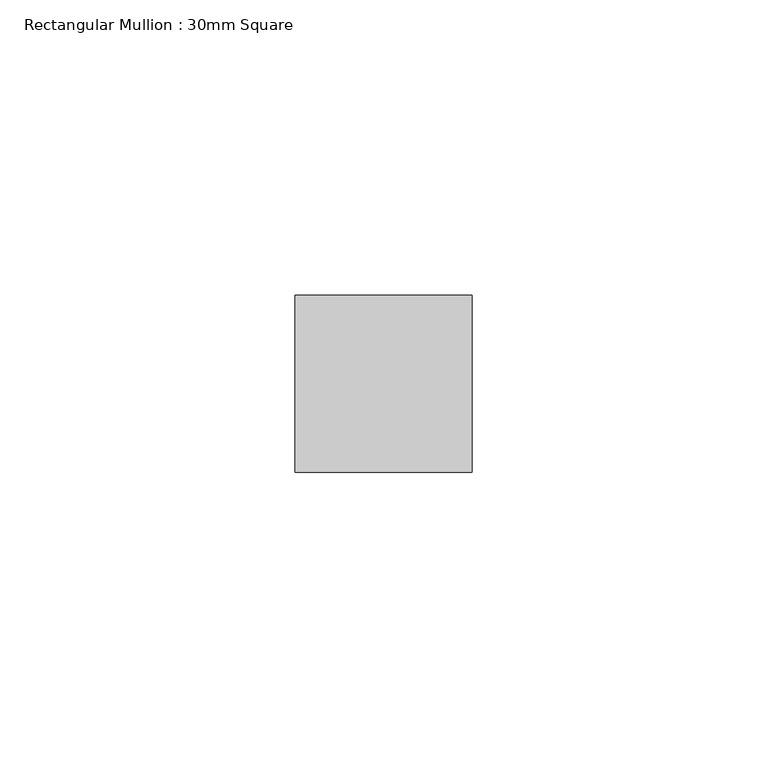
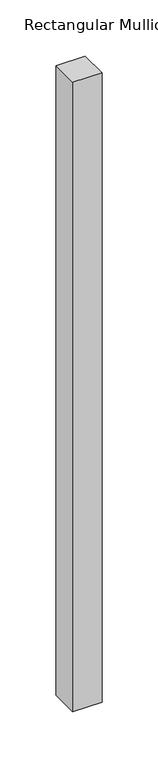
"""IFC4 building model written with IfcOpenShell, lengths in millimetres: member geometry, Rectangular Mullion : 30mm Square."""

from ifc_helpers import new_model, si_unit, frame, origin, place, context, project, spatial, polyline, outline, extrude, source, transform, mapped, element, save


def rectangular_mullion_30mm_square_3df302c3(model_context):
    return source(origin(), model_context, "Body", "SweptSolid", [
        extrude(outline(polyline([(15.0, 15.0), (15.0, -15.0), (-15.0, -15.0), (-15.0, 15.0), (15.0, 15.0)])), frame((0.0, 0.0, -685.0), z_axis=(0.0, 0.0, 1.0), x_axis=(1.0, 0.0, 0.0)), (0.0, 0.0, 1.0), 685.0),
    ])


if __name__ == "__main__":
    model = new_model("IFC4")
    model_context = context("Model", 3, world=origin())
    ifc_project = project(units=[si_unit("LENGTHUNIT", "METRE", prefix="MILLI")], contexts=[model_context])
    site = spatial("IfcSite", under=ifc_project)
    building = spatial("IfcBuilding", under=site)
    placement = place(None, origin())
    rectangular_mullion_30mm_square_shape = rectangular_mullion_30mm_square_3df302c3(model_context)
    element("IfcMember", 1, ObjectType="Rectangular Mullion : 30mm Square", at=placement, inside=building, context=model_context, shape_type="MappedRepresentation", body=[
        mapped(rectangular_mullion_30mm_square_shape, transform((0.0, 0.0, 0.0), x_axis=(1.0, 0.0, 0.0), y_axis=(0.0, 1.0, 0.0), z_axis=(0.0, 0.0, 1.0))),
    ])
    save(model, "model.ifc")

# Revit data of these elements
# Type "Rectangular Mullion : 30mm Square"
#   built-in parameter 1007304 = 0.0984252 (stored number, unit not read)
#   built-in parameter 1007301 = 0.0492126 (stored number, unit not read)
#   built-in parameter 1007300 = 0.0492126 (stored number, unit not read)
# Element 1 (IfcMember, "Rectangular Mullion : 30mm Square")
#   Materials on its faces: "Aluminum"
# Materials
#   "Aluminum": class "Metal", colour RGB 244 244 244, transparency 0, Description = "Aluminum 6061", Cost = 0
